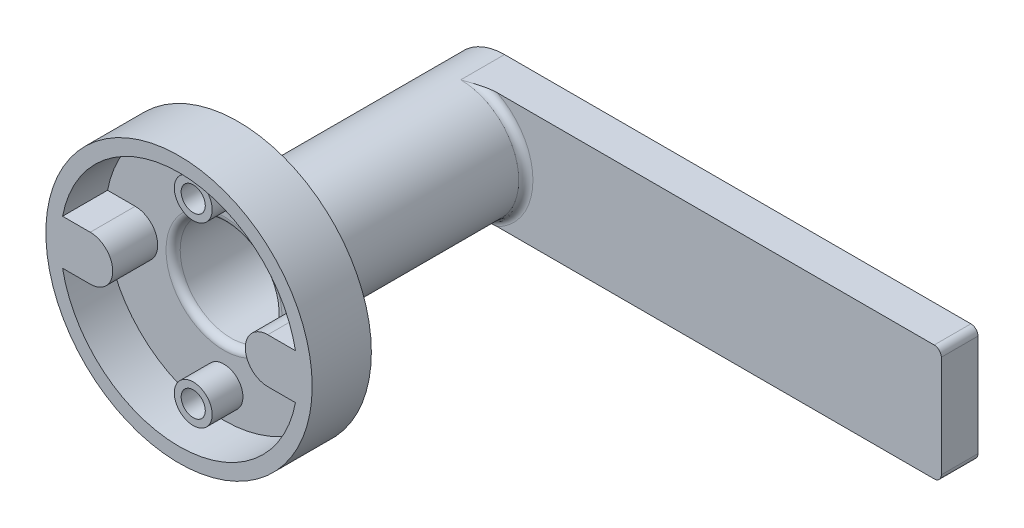
ISO-10303-21;
HEADER;
FILE_DESCRIPTION(('STEP AP214'),'2;1');
FILE_NAME('part.step','',(''),(''),'','','');
FILE_SCHEMA(('AUTOMOTIVE_DESIGN { 1 0 10303 214 1 1 1 1 }'));
ENDSEC;
DATA;
#1=APPLICATION_CONTEXT('core data for automotive mechanical design processes');
#2=APPLICATION_PROTOCOL_DEFINITION('international standard','automotive_design',2000,#1);
#3=PRODUCT_CONTEXT('',#1,'mechanical');
#4=PRODUCT('Part','Part','',(#3));
#5=PRODUCT_RELATED_PRODUCT_CATEGORY('part','',(#4));
#6=PRODUCT_DEFINITION_FORMATION('','',#4);
#7=PRODUCT_DEFINITION_CONTEXT('part definition',#1,'design');
#8=PRODUCT_DEFINITION('design','',#6,#7);
#9=PRODUCT_DEFINITION_SHAPE('','',#8);
#10=(LENGTH_UNIT() NAMED_UNIT(*) SI_UNIT(.MILLI.,.METRE.));
#11=(NAMED_UNIT(*) PLANE_ANGLE_UNIT() SI_UNIT($,.RADIAN.));
#12=(NAMED_UNIT(*) SI_UNIT($,.STERADIAN.) SOLID_ANGLE_UNIT());
#13=UNCERTAINTY_MEASURE_WITH_UNIT(LENGTH_MEASURE(1.E-05),#10,'distance_accuracy_value','');
#14=(GEOMETRIC_REPRESENTATION_CONTEXT(3) GLOBAL_UNCERTAINTY_ASSIGNED_CONTEXT((#13)) GLOBAL_UNIT_ASSIGNED_CONTEXT((#10,
#11,#12)) REPRESENTATION_CONTEXT('',''));
#15=CARTESIAN_POINT('',(0.,0.,0.));
#16=DIRECTION('',(0.,0.,1.));
#17=DIRECTION('',(1.,0.,0.));
#18=AXIS2_PLACEMENT_3D('',#15,#16,#17);
#19=CARTESIAN_POINT('',(0.,0.,12.7));
#20=DIRECTION('',(0.,0.,-1.));
#21=DIRECTION('',(-1.,0.,0.));
#22=AXIS2_PLACEMENT_3D('',#19,#20,#21);
#23=CYLINDRICAL_SURFACE('',#22,28.575);
#24=CARTESIAN_POINT('',(0.,0.,12.7));
#25=DIRECTION('',(0.,0.,1.));
#26=DIRECTION('',(1.,0.,0.));
#27=AXIS2_PLACEMENT_3D('',#24,#25,#26);
#28=CIRCLE('',#27,28.575);
#29=CARTESIAN_POINT('',(28.575,0.,12.7));
#30=VERTEX_POINT('',#29);
#31=EDGE_CURVE('E279',#30,#30,#28,.T.);
#32=ORIENTED_EDGE('',*,*,#31,.F.);
#33=EDGE_LOOP('',(#32));
#34=FACE_BOUND('',#33,.T.);
#35=CARTESIAN_POINT('',(0.,0.,0.));
#36=DIRECTION('',(0.,0.,1.));
#37=DIRECTION('',(1.,0.,0.));
#38=AXIS2_PLACEMENT_3D('',#35,#36,#37);
#39=CIRCLE('',#38,28.575);
#40=CARTESIAN_POINT('',(28.575,0.,0.));
#41=VERTEX_POINT('',#40);
#42=EDGE_CURVE('E263',#41,#41,#39,.T.);
#43=ORIENTED_EDGE('',*,*,#42,.T.);
#44=EDGE_LOOP('',(#43));
#45=FACE_BOUND('',#44,.T.);
#46=ADVANCED_FACE('F41',(#34,#45),#23,.T.);
#47=CARTESIAN_POINT('',(0.,0.,12.7));
#48=DIRECTION('',(0.,0.,1.));
#49=DIRECTION('',(1.,0.,0.));
#50=AXIS2_PLACEMENT_3D('',#47,#48,#49);
#51=PLANE('',#50);
#52=CARTESIAN_POINT('',(19.05,0.,12.7));
#53=DIRECTION('',(0.,0.,-1.));
#54=DIRECTION('',(-1.,0.,0.));
#55=AXIS2_PLACEMENT_3D('',#52,#53,#54);
#56=CIRCLE('',#55,4.826);
#57=CARTESIAN_POINT('',(19.05,-4.826,12.7));
#58=VERTEX_POINT('',#57);
#59=CARTESIAN_POINT('',(19.05,4.826,12.7));
#60=VERTEX_POINT('',#59);
#61=EDGE_CURVE('E214',#58,#60,#56,.T.);
#62=ORIENTED_EDGE('',*,*,#61,.F.);
#63=DIRECTION('',(-1.,0.,0.));
#64=VECTOR('',#63,1.);
#65=CARTESIAN_POINT('',(19.05,-4.826,12.7));
#66=LINE('',#65,#64);
#67=CARTESIAN_POINT('',(24.9900993985777,-4.826,12.7));
#68=VERTEX_POINT('',#67);
#69=EDGE_CURVE('E218',#68,#58,#66,.T.);
#70=ORIENTED_EDGE('',*,*,#69,.F.);
#71=CARTESIAN_POINT('',(0.,0.,12.7));
#72=DIRECTION('',(0.,0.,1.));
#73=DIRECTION('',(1.,0.,0.));
#74=AXIS2_PLACEMENT_3D('',#71,#72,#73);
#75=CIRCLE('',#74,25.451823980823);
#76=CARTESIAN_POINT('',(-24.9900993985777,-4.82599999999999,12.7));
#77=VERTEX_POINT('',#76);
#78=EDGE_CURVE('E257',#77,#68,#75,.T.);
#79=ORIENTED_EDGE('',*,*,#78,.F.);
#80=DIRECTION('',(-1.,0.,0.));
#81=VECTOR('',#80,1.);
#82=CARTESIAN_POINT('',(-19.05,-4.826,12.7));
#83=LINE('',#82,#81);
#84=CARTESIAN_POINT('',(-19.05,-4.826,12.7));
#85=VERTEX_POINT('',#84);
#86=EDGE_CURVE('E254',#85,#77,#83,.T.);
#87=ORIENTED_EDGE('',*,*,#86,.F.);
#88=CARTESIAN_POINT('',(-19.05,0.,12.7));
#89=DIRECTION('',(0.,0.,-1.));
#90=DIRECTION('',(1.,0.,0.));
#91=AXIS2_PLACEMENT_3D('',#88,#89,#90);
#92=CIRCLE('',#91,4.826);
#93=CARTESIAN_POINT('',(-19.05,4.826,12.7));
#94=VERTEX_POINT('',#93);
#95=EDGE_CURVE('E249',#94,#85,#92,.T.);
#96=ORIENTED_EDGE('',*,*,#95,.F.);
#97=DIRECTION('',(1.,0.,0.));
#98=VECTOR('',#97,1.);
#99=CARTESIAN_POINT('',(-19.05,4.826,12.7));
#100=LINE('',#99,#98);
#101=CARTESIAN_POINT('',(-24.9900993985777,4.826,12.7));
#102=VERTEX_POINT('',#101);
#103=EDGE_CURVE('E250',#102,#94,#100,.T.);
#104=ORIENTED_EDGE('',*,*,#103,.F.);
#105=CARTESIAN_POINT('',(0.,0.,12.7));
#106=DIRECTION('',(0.,0.,1.));
#107=DIRECTION('',(1.,0.,0.));
#108=AXIS2_PLACEMENT_3D('',#105,#106,#107);
#109=CIRCLE('',#108,25.451823980823);
#110=CARTESIAN_POINT('',(24.9900993985777,4.826,12.7));
#111=VERTEX_POINT('',#110);
#112=EDGE_CURVE('E242',#111,#102,#109,.T.);
#113=ORIENTED_EDGE('',*,*,#112,.F.);
#114=DIRECTION('',(1.,0.,0.));
#115=VECTOR('',#114,1.);
#116=CARTESIAN_POINT('',(19.05,4.826,12.7));
#117=LINE('',#116,#115);
#118=EDGE_CURVE('E241',#60,#111,#117,.T.);
#119=ORIENTED_EDGE('',*,*,#118,.F.);
#120=EDGE_LOOP('',(#62,#70,#79,#87,#96,#104,#113,#119));
#121=FACE_BOUND('',#120,.T.);
#122=ORIENTED_EDGE('',*,*,#31,.T.);
#123=EDGE_LOOP('',(#122));
#124=FACE_BOUND('',#123,.T.);
#125=ADVANCED_FACE('F344',(#121,#124),#51,.T.);
#126=CARTESIAN_POINT('',(0.,0.,0.));
#127=DIRECTION('',(0.,0.,1.));
#128=DIRECTION('',(1.,0.,0.));
#129=AXIS2_PLACEMENT_3D('',#126,#127,#128);
#130=PLANE('',#129);
#131=CARTESIAN_POINT('',(0.,0.,0.));
#132=DIRECTION('',(0.,0.,1.));
#133=DIRECTION('',(1.,0.,0.));
#134=AXIS2_PLACEMENT_3D('',#131,#132,#133);
#135=CIRCLE('',#134,12.446);
#136=CARTESIAN_POINT('',(12.446,0.,0.));
#137=VERTEX_POINT('',#136);
#138=EDGE_CURVE('E288',#137,#137,#135,.F.);
#139=ORIENTED_EDGE('',*,*,#138,.F.);
#140=EDGE_LOOP('',(#139));
#141=FACE_BOUND('',#140,.T.);
#142=CARTESIAN_POINT('',(0.,19.05,0.));
#143=DIRECTION('',(0.,0.,1.));
#144=DIRECTION('',(1.,0.,0.));
#145=AXIS2_PLACEMENT_3D('',#142,#143,#144);
#146=CIRCLE('',#145,2.59079999999999);
#147=CARTESIAN_POINT('',(2.59079999999999,19.05,0.));
#148=VERTEX_POINT('',#147);
#149=EDGE_CURVE('E198',#148,#148,#146,.T.);
#150=ORIENTED_EDGE('',*,*,#149,.T.);
#151=EDGE_LOOP('',(#150));
#152=FACE_BOUND('',#151,.T.);
#153=CARTESIAN_POINT('',(0.,-19.05,0.));
#154=DIRECTION('',(0.,0.,1.));
#155=DIRECTION('',(1.,0.,0.));
#156=AXIS2_PLACEMENT_3D('',#153,#154,#155);
#157=CIRCLE('',#156,2.59079999999999);
#158=CARTESIAN_POINT('',(2.59079999999999,-19.05,0.));
#159=VERTEX_POINT('',#158);
#160=EDGE_CURVE('E203',#159,#159,#157,.T.);
#161=ORIENTED_EDGE('',*,*,#160,.T.);
#162=EDGE_LOOP('',(#161));
#163=FACE_BOUND('',#162,.T.);
#164=ORIENTED_EDGE('',*,*,#42,.F.);
#165=EDGE_LOOP('',(#164));
#166=FACE_BOUND('',#165,.T.);
#167=ADVANCED_FACE('F348',(#141,#152,#163,#166),#130,.F.);
#168=CARTESIAN_POINT('',(19.05,0.,3.048));
#169=DIRECTION('',(0.,0.,1.));
#170=DIRECTION('',(1.,0.,0.));
#171=AXIS2_PLACEMENT_3D('',#168,#169,#170);
#172=CYLINDRICAL_SURFACE('',#171,4.826);
#173=ORIENTED_EDGE('',*,*,#61,.T.);
#174=DIRECTION('',(0.,0.,1.));
#175=VECTOR('',#174,1.);
#176=CARTESIAN_POINT('',(19.05,4.826,3.048));
#177=LINE('',#176,#175);
#178=CARTESIAN_POINT('',(19.05,4.826,3.048));
#179=VERTEX_POINT('',#178);
#180=EDGE_CURVE('E237',#179,#60,#177,.T.);
#181=ORIENTED_EDGE('',*,*,#180,.F.);
#182=CARTESIAN_POINT('',(19.05,0.,3.048));
#183=DIRECTION('',(0.,0.,-1.));
#184=DIRECTION('',(-1.,0.,0.));
#185=AXIS2_PLACEMENT_3D('',#182,#183,#184);
#186=CIRCLE('',#185,4.826);
#187=CARTESIAN_POINT('',(19.05,-4.826,3.048));
#188=VERTEX_POINT('',#187);
#189=EDGE_CURVE('E211',#188,#179,#186,.T.);
#190=ORIENTED_EDGE('',*,*,#189,.F.);
#191=DIRECTION('',(0.,0.,1.));
#192=VECTOR('',#191,1.);
#193=CARTESIAN_POINT('',(19.05,-4.826,3.048));
#194=LINE('',#193,#192);
#195=EDGE_CURVE('E262',#188,#58,#194,.T.);
#196=ORIENTED_EDGE('',*,*,#195,.T.);
#197=EDGE_LOOP('',(#173,#181,#190,#196));
#198=FACE_BOUND('',#197,.T.);
#199=ADVANCED_FACE('F358',(#198),#172,.T.);
#200=CARTESIAN_POINT('',(19.05,-4.826,3.048));
#201=DIRECTION('',(0.,1.,0.));
#202=DIRECTION('',(-1.,0.,0.));
#203=AXIS2_PLACEMENT_3D('',#200,#201,#202);
#204=PLANE('',#203);
#205=ORIENTED_EDGE('',*,*,#69,.T.);
#206=ORIENTED_EDGE('',*,*,#195,.F.);
#207=DIRECTION('',(-1.,0.,0.));
#208=VECTOR('',#207,1.);
#209=CARTESIAN_POINT('',(19.05,-4.826,3.048));
#210=LINE('',#209,#208);
#211=CARTESIAN_POINT('',(24.9900993985777,-4.826,3.048));
#212=VERTEX_POINT('',#211);
#213=EDGE_CURVE('E236',#212,#188,#210,.T.);
#214=ORIENTED_EDGE('',*,*,#213,.F.);
#215=DIRECTION('',(0.,0.,1.));
#216=VECTOR('',#215,1.);
#217=CARTESIAN_POINT('',(24.9900993985777,-4.826,3.048));
#218=LINE('',#217,#216);
#219=EDGE_CURVE('E264',#212,#68,#218,.T.);
#220=ORIENTED_EDGE('',*,*,#219,.T.);
#221=EDGE_LOOP('',(#205,#206,#214,#220));
#222=FACE_BOUND('',#221,.T.);
#223=ADVANCED_FACE('F361',(#222),#204,.F.);
#224=CARTESIAN_POINT('',(0.,0.,3.048));
#225=DIRECTION('',(0.,0.,1.));
#226=DIRECTION('',(1.,0.,0.));
#227=AXIS2_PLACEMENT_3D('',#224,#225,#226);
#228=CYLINDRICAL_SURFACE('',#227,25.451823980823);
#229=ORIENTED_EDGE('',*,*,#78,.T.);
#230=ORIENTED_EDGE('',*,*,#219,.F.);
#231=CARTESIAN_POINT('',(0.,0.,3.048));
#232=DIRECTION('',(0.,0.,1.));
#233=DIRECTION('',(1.,0.,0.));
#234=AXIS2_PLACEMENT_3D('',#231,#232,#233);
#235=CIRCLE('',#234,25.451823980823);
#236=CARTESIAN_POINT('',(-24.9900993985777,-4.82599999999999,3.048));
#237=VERTEX_POINT('',#236);
#238=EDGE_CURVE('E231',#237,#212,#235,.T.);
#239=ORIENTED_EDGE('',*,*,#238,.F.);
#240=DIRECTION('',(0.,0.,1.));
#241=VECTOR('',#240,1.);
#242=CARTESIAN_POINT('',(-24.9900993985777,-4.82599999999999,3.048));
#243=LINE('',#242,#241);
#244=EDGE_CURVE('E269',#237,#77,#243,.T.);
#245=ORIENTED_EDGE('',*,*,#244,.T.);
#246=EDGE_LOOP('',(#229,#230,#239,#245));
#247=FACE_BOUND('',#246,.T.);
#248=ADVANCED_FACE('F386',(#247),#228,.F.);
#249=CARTESIAN_POINT('',(-19.05,-4.826,3.048));
#250=DIRECTION('',(0.,1.,0.));
#251=DIRECTION('',(-1.,0.,0.));
#252=AXIS2_PLACEMENT_3D('',#249,#250,#251);
#253=PLANE('',#252);
#254=ORIENTED_EDGE('',*,*,#86,.T.);
#255=ORIENTED_EDGE('',*,*,#244,.F.);
#256=DIRECTION('',(-1.,0.,0.));
#257=VECTOR('',#256,1.);
#258=CARTESIAN_POINT('',(-19.05,-4.826,3.048));
#259=LINE('',#258,#257);
#260=CARTESIAN_POINT('',(-19.05,-4.826,3.048));
#261=VERTEX_POINT('',#260);
#262=EDGE_CURVE('E229',#261,#237,#259,.T.);
#263=ORIENTED_EDGE('',*,*,#262,.F.);
#264=DIRECTION('',(0.,0.,1.));
#265=VECTOR('',#264,1.);
#266=CARTESIAN_POINT('',(-19.05,-4.826,3.048));
#267=LINE('',#266,#265);
#268=EDGE_CURVE('E270',#261,#85,#267,.T.);
#269=ORIENTED_EDGE('',*,*,#268,.T.);
#270=EDGE_LOOP('',(#254,#255,#263,#269));
#271=FACE_BOUND('',#270,.T.);
#272=ADVANCED_FACE('F383',(#271),#253,.F.);
#273=CARTESIAN_POINT('',(-19.05,0.,3.048));
#274=DIRECTION('',(0.,0.,1.));
#275=DIRECTION('',(1.,0.,0.));
#276=AXIS2_PLACEMENT_3D('',#273,#274,#275);
#277=CYLINDRICAL_SURFACE('',#276,4.826);
#278=ORIENTED_EDGE('',*,*,#95,.T.);
#279=ORIENTED_EDGE('',*,*,#268,.F.);
#280=CARTESIAN_POINT('',(-19.05,0.,3.048));
#281=DIRECTION('',(0.,0.,-1.));
#282=DIRECTION('',(1.,0.,0.));
#283=AXIS2_PLACEMENT_3D('',#280,#281,#282);
#284=CIRCLE('',#283,4.826);
#285=CARTESIAN_POINT('',(-19.05,4.826,3.048));
#286=VERTEX_POINT('',#285);
#287=EDGE_CURVE('E227',#286,#261,#284,.T.);
#288=ORIENTED_EDGE('',*,*,#287,.F.);
#289=DIRECTION('',(0.,0.,1.));
#290=VECTOR('',#289,1.);
#291=CARTESIAN_POINT('',(-19.05,4.826,3.048));
#292=LINE('',#291,#290);
#293=EDGE_CURVE('E267',#286,#94,#292,.T.);
#294=ORIENTED_EDGE('',*,*,#293,.T.);
#295=EDGE_LOOP('',(#278,#279,#288,#294));
#296=FACE_BOUND('',#295,.T.);
#297=ADVANCED_FACE('F382',(#296),#277,.T.);
#298=CARTESIAN_POINT('',(-19.05,4.826,3.048));
#299=DIRECTION('',(0.,-1.,0.));
#300=DIRECTION('',(1.,0.,0.));
#301=AXIS2_PLACEMENT_3D('',#298,#299,#300);
#302=PLANE('',#301);
#303=ORIENTED_EDGE('',*,*,#103,.T.);
#304=ORIENTED_EDGE('',*,*,#293,.F.);
#305=DIRECTION('',(1.,0.,0.));
#306=VECTOR('',#305,1.);
#307=CARTESIAN_POINT('',(-19.05,4.826,3.048));
#308=LINE('',#307,#306);
#309=CARTESIAN_POINT('',(-24.9900993985777,4.826,3.048));
#310=VERTEX_POINT('',#309);
#311=EDGE_CURVE('E223',#310,#286,#308,.T.);
#312=ORIENTED_EDGE('',*,*,#311,.F.);
#313=DIRECTION('',(0.,0.,1.));
#314=VECTOR('',#313,1.);
#315=CARTESIAN_POINT('',(-24.9900993985777,4.826,3.048));
#316=LINE('',#315,#314);
#317=EDGE_CURVE('E275',#310,#102,#316,.T.);
#318=ORIENTED_EDGE('',*,*,#317,.T.);
#319=EDGE_LOOP('',(#303,#304,#312,#318));
#320=FACE_BOUND('',#319,.T.);
#321=ADVANCED_FACE('F380',(#320),#302,.F.);
#322=CARTESIAN_POINT('',(0.,0.,3.048));
#323=DIRECTION('',(0.,0.,1.));
#324=DIRECTION('',(1.,0.,0.));
#325=AXIS2_PLACEMENT_3D('',#322,#323,#324);
#326=CYLINDRICAL_SURFACE('',#325,25.451823980823);
#327=ORIENTED_EDGE('',*,*,#112,.T.);
#328=ORIENTED_EDGE('',*,*,#317,.F.);
#329=CARTESIAN_POINT('',(0.,0.,3.048));
#330=DIRECTION('',(0.,0.,1.));
#331=DIRECTION('',(1.,0.,0.));
#332=AXIS2_PLACEMENT_3D('',#329,#330,#331);
#333=CIRCLE('',#332,25.451823980823);
#334=CARTESIAN_POINT('',(24.9900993985777,4.826,3.048));
#335=VERTEX_POINT('',#334);
#336=EDGE_CURVE('E224',#335,#310,#333,.T.);
#337=ORIENTED_EDGE('',*,*,#336,.F.);
#338=DIRECTION('',(0.,0.,1.));
#339=VECTOR('',#338,1.);
#340=CARTESIAN_POINT('',(24.9900993985777,4.826,3.048));
#341=LINE('',#340,#339);
#342=EDGE_CURVE('E274',#335,#111,#341,.T.);
#343=ORIENTED_EDGE('',*,*,#342,.T.);
#344=EDGE_LOOP('',(#327,#328,#337,#343));
#345=FACE_BOUND('',#344,.T.);
#346=ADVANCED_FACE('F373',(#345),#326,.F.);
#347=CARTESIAN_POINT('',(19.05,4.826,3.048));
#348=DIRECTION('',(0.,-1.,0.));
#349=DIRECTION('',(1.,0.,0.));
#350=AXIS2_PLACEMENT_3D('',#347,#348,#349);
#351=PLANE('',#350);
#352=ORIENTED_EDGE('',*,*,#118,.T.);
#353=ORIENTED_EDGE('',*,*,#342,.F.);
#354=DIRECTION('',(1.,0.,0.));
#355=VECTOR('',#354,1.);
#356=CARTESIAN_POINT('',(19.05,4.826,3.048));
#357=LINE('',#356,#355);
#358=EDGE_CURVE('E220',#179,#335,#357,.T.);
#359=ORIENTED_EDGE('',*,*,#358,.F.);
#360=ORIENTED_EDGE('',*,*,#180,.T.);
#361=EDGE_LOOP('',(#352,#353,#359,#360));
#362=FACE_BOUND('',#361,.T.);
#363=ADVANCED_FACE('F367',(#362),#351,.F.);
#364=CARTESIAN_POINT('',(19.05,0.,3.048));
#365=DIRECTION('',(0.,0.,-1.));
#366=DIRECTION('',(-1.,0.,0.));
#367=AXIS2_PLACEMENT_3D('',#364,#365,#366);
#368=PLANE('',#367);
#369=CARTESIAN_POINT('',(0.,0.,3.048));
#370=DIRECTION('',(0.,0.,-1.));
#371=DIRECTION('',(-1.,0.,0.));
#372=AXIS2_PLACEMENT_3D('',#369,#370,#371);
#373=CIRCLE('',#372,12.446);
#374=CARTESIAN_POINT('',(-12.446,0.,3.048));
#375=VERTEX_POINT('',#374);
#376=EDGE_CURVE('E302',#375,#375,#373,.T.);
#377=ORIENTED_EDGE('',*,*,#376,.T.);
#378=EDGE_LOOP('',(#377));
#379=FACE_BOUND('',#378,.T.);
#380=CARTESIAN_POINT('',(0.,-19.05,3.048));
#381=DIRECTION('',(0.,0.,-1.));
#382=DIRECTION('',(-1.,0.,0.));
#383=AXIS2_PLACEMENT_3D('',#380,#381,#382);
#384=CIRCLE('',#383,4.064);
#385=CARTESIAN_POINT('',(-4.064,-19.05,3.048));
#386=VERTEX_POINT('',#385);
#387=EDGE_CURVE('E289',#386,#386,#384,.F.);
#388=ORIENTED_EDGE('',*,*,#387,.F.);
#389=EDGE_LOOP('',(#388));
#390=FACE_BOUND('',#389,.T.);
#391=CARTESIAN_POINT('',(0.,19.05,3.048));
#392=DIRECTION('',(0.,0.,-1.));
#393=DIRECTION('',(-1.,0.,0.));
#394=AXIS2_PLACEMENT_3D('',#391,#392,#393);
#395=CIRCLE('',#394,4.064);
#396=CARTESIAN_POINT('',(-4.064,19.05,3.048));
#397=VERTEX_POINT('',#396);
#398=EDGE_CURVE('E282',#397,#397,#395,.F.);
#399=ORIENTED_EDGE('',*,*,#398,.F.);
#400=EDGE_LOOP('',(#399));
#401=FACE_BOUND('',#400,.T.);
#402=ORIENTED_EDGE('',*,*,#189,.T.);
#403=ORIENTED_EDGE('',*,*,#358,.T.);
#404=ORIENTED_EDGE('',*,*,#336,.T.);
#405=ORIENTED_EDGE('',*,*,#311,.T.);
#406=ORIENTED_EDGE('',*,*,#287,.T.);
#407=ORIENTED_EDGE('',*,*,#262,.T.);
#408=ORIENTED_EDGE('',*,*,#238,.T.);
#409=ORIENTED_EDGE('',*,*,#213,.T.);
#410=EDGE_LOOP('',(#402,#403,#404,#405,#406,#407,#408,#409));
#411=FACE_BOUND('',#410,.T.);
#412=ADVANCED_FACE('F375',(#379,#390,#401,#411),#368,.F.);
#413=CARTESIAN_POINT('',(0.,19.05,24.1947278349685));
#414=DIRECTION('',(0.,0.,-1.));
#415=DIRECTION('',(-1.,0.,0.));
#416=AXIS2_PLACEMENT_3D('',#413,#414,#415);
#417=CYLINDRICAL_SURFACE('',#416,4.064);
#418=ORIENTED_EDGE('',*,*,#398,.T.);
#419=EDGE_LOOP('',(#418));
#420=FACE_BOUND('',#419,.T.);
#421=CARTESIAN_POINT('',(0.,19.05,9.652));
#422=DIRECTION('',(0.,0.,1.));
#423=DIRECTION('',(1.,0.,0.));
#424=AXIS2_PLACEMENT_3D('',#421,#422,#423);
#425=CIRCLE('',#424,4.064);
#426=CARTESIAN_POINT('',(4.064,19.05,9.652));
#427=VERTEX_POINT('',#426);
#428=EDGE_CURVE('E208',#427,#427,#425,.T.);
#429=ORIENTED_EDGE('',*,*,#428,.F.);
#430=EDGE_LOOP('',(#429));
#431=FACE_BOUND('',#430,.T.);
#432=ADVANCED_FACE('F398',(#420,#431),#417,.T.);
#433=CARTESIAN_POINT('',(0.,0.,9.652));
#434=DIRECTION('',(0.,0.,1.));
#435=DIRECTION('',(1.,0.,0.));
#436=AXIS2_PLACEMENT_3D('',#433,#434,#435);
#437=PLANE('',#436);
#438=CARTESIAN_POINT('',(0.,19.05,9.652));
#439=DIRECTION('',(0.,0.,1.));
#440=DIRECTION('',(1.,0.,0.));
#441=AXIS2_PLACEMENT_3D('',#438,#439,#440);
#442=CIRCLE('',#441,2.59079999999999);
#443=CARTESIAN_POINT('',(2.59079999999999,19.05,9.652));
#444=VERTEX_POINT('',#443);
#445=EDGE_CURVE('E193',#444,#444,#442,.T.);
#446=ORIENTED_EDGE('',*,*,#445,.F.);
#447=EDGE_LOOP('',(#446));
#448=FACE_BOUND('',#447,.T.);
#449=ORIENTED_EDGE('',*,*,#428,.T.);
#450=EDGE_LOOP('',(#449));
#451=FACE_BOUND('',#450,.T.);
#452=ADVANCED_FACE('F402',(#448,#451),#437,.T.);
#453=CARTESIAN_POINT('',(0.,-19.05,24.1947278349685));
#454=DIRECTION('',(0.,0.,-1.));
#455=DIRECTION('',(-1.,0.,0.));
#456=AXIS2_PLACEMENT_3D('',#453,#454,#455);
#457=CYLINDRICAL_SURFACE('',#456,4.064);
#458=ORIENTED_EDGE('',*,*,#387,.T.);
#459=EDGE_LOOP('',(#458));
#460=FACE_BOUND('',#459,.T.);
#461=CARTESIAN_POINT('',(0.,-19.05,9.652));
#462=DIRECTION('',(0.,0.,1.));
#463=DIRECTION('',(1.,0.,0.));
#464=AXIS2_PLACEMENT_3D('',#461,#462,#463);
#465=CIRCLE('',#464,4.064);
#466=CARTESIAN_POINT('',(4.064,-19.05,9.652));
#467=VERTEX_POINT('',#466);
#468=EDGE_CURVE('E210',#467,#467,#465,.T.);
#469=ORIENTED_EDGE('',*,*,#468,.F.);
#470=EDGE_LOOP('',(#469));
#471=FACE_BOUND('',#470,.T.);
#472=ADVANCED_FACE('F404',(#460,#471),#457,.T.);
#473=CARTESIAN_POINT('',(0.,0.,9.652));
#474=DIRECTION('',(0.,0.,1.));
#475=DIRECTION('',(1.,0.,0.));
#476=AXIS2_PLACEMENT_3D('',#473,#474,#475);
#477=PLANE('',#476);
#478=CARTESIAN_POINT('',(0.,-19.05,9.652));
#479=DIRECTION('',(0.,0.,1.));
#480=DIRECTION('',(1.,0.,0.));
#481=AXIS2_PLACEMENT_3D('',#478,#479,#480);
#482=CIRCLE('',#481,2.59079999999999);
#483=CARTESIAN_POINT('',(2.59079999999999,-19.05,9.652));
#484=VERTEX_POINT('',#483);
#485=EDGE_CURVE('E204',#484,#484,#482,.T.);
#486=ORIENTED_EDGE('',*,*,#485,.F.);
#487=EDGE_LOOP('',(#486));
#488=FACE_BOUND('',#487,.T.);
#489=ORIENTED_EDGE('',*,*,#468,.T.);
#490=EDGE_LOOP('',(#489));
#491=FACE_BOUND('',#490,.T.);
#492=ADVANCED_FACE('F406',(#488,#491),#477,.T.);
#493=CARTESIAN_POINT('',(0.,-19.05,9.652));
#494=DIRECTION('',(0.,0.,1.));
#495=DIRECTION('',(1.,0.,0.));
#496=AXIS2_PLACEMENT_3D('',#493,#494,#495);
#497=CYLINDRICAL_SURFACE('',#496,2.59079999999999);
#498=ORIENTED_EDGE('',*,*,#485,.T.);
#499=EDGE_LOOP('',(#498));
#500=FACE_BOUND('',#499,.T.);
#501=ORIENTED_EDGE('',*,*,#160,.F.);
#502=EDGE_LOOP('',(#501));
#503=FACE_BOUND('',#502,.T.);
#504=ADVANCED_FACE('F415',(#500,#503),#497,.F.);
#505=CARTESIAN_POINT('',(0.,19.05,9.652));
#506=DIRECTION('',(0.,0.,1.));
#507=DIRECTION('',(1.,0.,0.));
#508=AXIS2_PLACEMENT_3D('',#505,#506,#507);
#509=CYLINDRICAL_SURFACE('',#508,2.59079999999999);
#510=ORIENTED_EDGE('',*,*,#445,.T.);
#511=EDGE_LOOP('',(#510));
#512=FACE_BOUND('',#511,.T.);
#513=ORIENTED_EDGE('',*,*,#149,.F.);
#514=EDGE_LOOP('',(#513));
#515=FACE_BOUND('',#514,.T.);
#516=ADVANCED_FACE('F418',(#512,#515),#509,.F.);
#517=CARTESIAN_POINT('',(0.,0.,-49.276));
#518=DIRECTION('',(0.,0.,1.));
#519=DIRECTION('',(1.,0.,0.));
#520=AXIS2_PLACEMENT_3D('',#517,#518,#519);
#521=CYLINDRICAL_SURFACE('',#520,12.446);
#522=DIRECTION('',(0.,0.,1.));
#523=VECTOR('',#522,1.);
#524=CARTESIAN_POINT('',(0.,-12.446,-57.15));
#525=LINE('',#524,#523);
#526=CARTESIAN_POINT('',(0.,-12.446,-57.15));
#527=VERTEX_POINT('',#526);
#528=CARTESIAN_POINT('',(0.,-12.446,-47.752));
#529=VERTEX_POINT('',#528);
#530=EDGE_CURVE('E167',#527,#529,#525,.T.);
#531=ORIENTED_EDGE('',*,*,#530,.T.);
#532=CARTESIAN_POINT('',(0.,0.,-47.752));
#533=DIRECTION('',(0.,0.,-1.));
#534=DIRECTION('',(-1.,0.,0.));
#535=AXIS2_PLACEMENT_3D('',#532,#533,#534);
#536=CIRCLE('',#535,12.446);
#537=CARTESIAN_POINT('',(0.,12.446,-47.752));
#538=VERTEX_POINT('',#537);
#539=EDGE_CURVE('E299',#529,#538,#536,.F.);
#540=ORIENTED_EDGE('',*,*,#539,.T.);
#541=DIRECTION('',(0.,0.,1.));
#542=VECTOR('',#541,1.);
#543=CARTESIAN_POINT('',(0.,12.446,-57.15));
#544=LINE('',#543,#542);
#545=CARTESIAN_POINT('',(0.,12.446,-57.15));
#546=VERTEX_POINT('',#545);
#547=EDGE_CURVE('E180',#546,#538,#544,.T.);
#548=ORIENTED_EDGE('',*,*,#547,.F.);
#549=CARTESIAN_POINT('',(0.,0.,-57.15));
#550=DIRECTION('',(0.,0.,-1.));
#551=DIRECTION('',(-1.,0.,0.));
#552=AXIS2_PLACEMENT_3D('',#549,#550,#551);
#553=CIRCLE('',#552,12.446);
#554=EDGE_CURVE('E157',#527,#546,#553,.T.);
#555=ORIENTED_EDGE('',*,*,#554,.F.);
#556=EDGE_LOOP('',(#531,#540,#548,#555));
#557=FACE_BOUND('',#556,.T.);
#558=ORIENTED_EDGE('',*,*,#138,.T.);
#559=EDGE_LOOP('',(#558));
#560=FACE_BOUND('',#559,.T.);
#561=ADVANCED_FACE('F177',(#557,#560),#521,.T.);
#562=CARTESIAN_POINT('',(0.,0.,-80.1680810564779));
#563=DIRECTION('',(0.,0.,1.));
#564=DIRECTION('',(1.,0.,0.));
#565=AXIS2_PLACEMENT_3D('',#562,#563,#564);
#566=CYLINDRICAL_SURFACE('',#565,10.922);
#567=CARTESIAN_POINT('',(0.,0.,1.524));
#568=DIRECTION('',(0.,0.,-1.));
#569=DIRECTION('',(-1.,0.,0.));
#570=AXIS2_PLACEMENT_3D('',#567,#568,#569);
#571=CIRCLE('',#570,10.922);
#572=CARTESIAN_POINT('',(-10.922,0.,1.524));
#573=VERTEX_POINT('',#572);
#574=EDGE_CURVE('E301',#573,#573,#571,.F.);
#575=ORIENTED_EDGE('',*,*,#574,.T.);
#576=EDGE_LOOP('',(#575));
#577=FACE_BOUND('',#576,.T.);
#578=CARTESIAN_POINT('',(0.,0.,-49.276));
#579=DIRECTION('',(0.,0.,-1.));
#580=DIRECTION('',(-1.,0.,0.));
#581=AXIS2_PLACEMENT_3D('',#578,#579,#580);
#582=CIRCLE('',#581,10.922);
#583=CARTESIAN_POINT('',(-10.922,0.,-49.276));
#584=VERTEX_POINT('',#583);
#585=EDGE_CURVE('E176',#584,#584,#582,.F.);
#586=ORIENTED_EDGE('',*,*,#585,.F.);
#587=EDGE_LOOP('',(#586));
#588=FACE_BOUND('',#587,.T.);
#589=ADVANCED_FACE('F424',(#577,#588),#566,.F.);
#590=CARTESIAN_POINT('',(0.,0.,-57.15));
#591=DIRECTION('',(0.,0.,-1.));
#592=DIRECTION('',(-1.,0.,0.));
#593=AXIS2_PLACEMENT_3D('',#590,#591,#592);
#594=PLANE('',#593);
#595=DIRECTION('',(0.,-1.,0.));
#596=VECTOR('',#595,1.);
#597=CARTESIAN_POINT('',(101.6,12.446,-57.15));
#598=LINE('',#597,#596);
#599=CARTESIAN_POINT('',(101.6,10.922,-57.15));
#600=VERTEX_POINT('',#599);
#601=CARTESIAN_POINT('',(101.6,-10.922,-57.15));
#602=VERTEX_POINT('',#601);
#603=EDGE_CURVE('E170',#600,#602,#598,.T.);
#604=ORIENTED_EDGE('',*,*,#603,.T.);
#605=CARTESIAN_POINT('',(100.076,-10.922,-57.15));
#606=DIRECTION('',(0.,0.,-1.));
#607=DIRECTION('',(-1.,0.,0.));
#608=AXIS2_PLACEMENT_3D('',#605,#606,#607);
#609=CIRCLE('',#608,1.524);
#610=CARTESIAN_POINT('',(100.076,-12.446,-57.15));
#611=VERTEX_POINT('',#610);
#612=EDGE_CURVE('E161',#602,#611,#609,.T.);
#613=ORIENTED_EDGE('',*,*,#612,.T.);
#614=DIRECTION('',(-1.,0.,0.));
#615=VECTOR('',#614,1.);
#616=CARTESIAN_POINT('',(101.6,-12.446,-57.15));
#617=LINE('',#616,#615);
#618=EDGE_CURVE('E159',#611,#527,#617,.T.);
#619=ORIENTED_EDGE('',*,*,#618,.T.);
#620=ORIENTED_EDGE('',*,*,#554,.T.);
#621=DIRECTION('',(1.,0.,0.));
#622=VECTOR('',#621,1.);
#623=CARTESIAN_POINT('',(101.6,12.446,-57.15));
#624=LINE('',#623,#622);
#625=CARTESIAN_POINT('',(100.076,12.446,-57.15));
#626=VERTEX_POINT('',#625);
#627=EDGE_CURVE('E181',#546,#626,#624,.T.);
#628=ORIENTED_EDGE('',*,*,#627,.T.);
#629=CARTESIAN_POINT('',(100.076,10.922,-57.15));
#630=DIRECTION('',(0.,0.,-1.));
#631=DIRECTION('',(-1.,0.,0.));
#632=AXIS2_PLACEMENT_3D('',#629,#630,#631);
#633=CIRCLE('',#632,1.524);
#634=EDGE_CURVE('E312',#626,#600,#633,.T.);
#635=ORIENTED_EDGE('',*,*,#634,.T.);
#636=EDGE_LOOP('',(#604,#613,#619,#620,#628,#635));
#637=FACE_BOUND('',#636,.T.);
#638=ADVANCED_FACE('F160',(#637),#594,.T.);
#639=CARTESIAN_POINT('',(101.6,12.446,-57.15));
#640=DIRECTION('',(0.,-1.,0.));
#641=DIRECTION('',(0.,0.,-1.));
#642=AXIS2_PLACEMENT_3D('',#639,#640,#641);
#643=PLANE('',#642);
#644=DIRECTION('',(1.,0.,0.));
#645=VECTOR('',#644,1.);
#646=CARTESIAN_POINT('',(101.6,12.446,-49.276));
#647=LINE('',#646,#645);
#648=CARTESIAN_POINT('',(6.34491796637277,12.446,-49.276));
#649=VERTEX_POINT('',#648);
#650=CARTESIAN_POINT('',(100.076,12.446,-49.276));
#651=VERTEX_POINT('',#650);
#652=EDGE_CURVE('E188',#649,#651,#647,.T.);
#653=ORIENTED_EDGE('',*,*,#652,.T.);
#654=DIRECTION('',(0.,0.,1.));
#655=VECTOR('',#654,1.);
#656=CARTESIAN_POINT('',(100.076,12.446,-57.15));
#657=LINE('',#656,#655);
#658=EDGE_CURVE('E65',#651,#626,#657,.F.);
#659=ORIENTED_EDGE('',*,*,#658,.T.);
#660=ORIENTED_EDGE('',*,*,#627,.F.);
#661=ORIENTED_EDGE('',*,*,#547,.T.);
#662=CARTESIAN_POINT('',(6.34491796637277,12.446,-49.276));
#663=CARTESIAN_POINT('',(6.21533524094485,12.446,-49.2759732705405));
#664=CARTESIAN_POINT('',(6.08579369063811,12.446,-49.27259226928));
#665=CARTESIAN_POINT('',(5.82706524459241,12.446,-49.259910087951));
#666=CARTESIAN_POINT('',(5.6978781945778,12.446,-49.2506121205866));
#667=CARTESIAN_POINT('',(5.4402955593906,12.446,-49.2269107528351));
#668=CARTESIAN_POINT('',(5.31189882415412,12.446,-49.2125195023357));
#669=CARTESIAN_POINT('',(5.05567590714475,12.446,-49.1792496205522));
#670=CARTESIAN_POINT('',(4.92784981517291,12.446,-49.1603703067066));
#671=CARTESIAN_POINT('',(4.54726190236325,12.446,-49.0981575716032));
#672=CARTESIAN_POINT('',(4.29543863295937,12.446,-49.0490520465874));
#673=CARTESIAN_POINT('',(3.79431096207436,12.446,-48.9389015359754));
#674=CARTESIAN_POINT('',(3.54500841851374,12.446,-48.8778483354951));
#675=CARTESIAN_POINT('',(3.01979635859548,12.446,-48.7389881468602));
#676=CARTESIAN_POINT('',(2.74418711385954,12.446,-48.6600566773526));
#677=CARTESIAN_POINT('',(2.19547772469525,12.446,-48.4941969315973));
#678=CARTESIAN_POINT('',(1.92237711929461,12.446,-48.4072701582111));
#679=CARTESIAN_POINT('',(1.1047936535399,12.446,-48.1385183371954));
#680=CARTESIAN_POINT('',(0.562885676700975,12.446,-47.9489679517187));
#681=CARTESIAN_POINT('',(0.0140400977837042,12.446,-47.7569129993086));
#682=CARTESIAN_POINT('',(0.00702004561032453,12.446,-47.7544564925513));
#683=CARTESIAN_POINT('',(0.,12.446,-47.752));
#684=B_SPLINE_CURVE_WITH_KNOTS('',3,(#662,#663,#664,#665,#666,#667,#668,#669,#670,#671,#672,
#673,#674,#675,#676,#677,#678,#679,#680,#681,#682,#683),.UNSPECIFIED.,.F.,.F.,(4,2,2,2,2,2,2,2,
2,2,4),(0.,0.388645930924585,0.777081020636638,1.16459568621553,1.5521693242234,
2.32144242636155,3.09124632924267,3.95113147757733,4.81085532404043,6.5329742853189,
6.5552866137498),.UNSPECIFIED.);
#685=EDGE_CURVE('E12',#538,#649,#684,.F.);
#686=ORIENTED_EDGE('',*,*,#685,.T.);
#687=EDGE_LOOP('',(#653,#659,#660,#661,#686));
#688=FACE_BOUND('',#687,.T.);
#689=ADVANCED_FACE('F440',(#688),#643,.F.);
#690=CARTESIAN_POINT('',(101.6,-12.446,-57.15));
#691=DIRECTION('',(0.,1.,0.));
#692=DIRECTION('',(0.,0.,1.));
#693=AXIS2_PLACEMENT_3D('',#690,#691,#692);
#694=PLANE('',#693);
#695=ORIENTED_EDGE('',*,*,#618,.F.);
#696=DIRECTION('',(0.,0.,1.));
#697=VECTOR('',#696,1.);
#698=CARTESIAN_POINT('',(100.076,-12.446,-57.15));
#699=LINE('',#698,#697);
#700=CARTESIAN_POINT('',(100.076,-12.446,-49.276));
#701=VERTEX_POINT('',#700);
#702=EDGE_CURVE('E310',#611,#701,#699,.T.);
#703=ORIENTED_EDGE('',*,*,#702,.T.);
#704=DIRECTION('',(-1.,0.,0.));
#705=VECTOR('',#704,1.);
#706=CARTESIAN_POINT('',(101.6,-12.446,-49.276));
#707=LINE('',#706,#705);
#708=CARTESIAN_POINT('',(6.34491796637277,-12.446,-49.276));
#709=VERTEX_POINT('',#708);
#710=EDGE_CURVE('E189',#701,#709,#707,.T.);
#711=ORIENTED_EDGE('',*,*,#710,.T.);
#712=CARTESIAN_POINT('',(6.34491796637277,-12.446,-49.276));
#713=CARTESIAN_POINT('',(6.21533524094485,-12.446,-49.2759732705405));
#714=CARTESIAN_POINT('',(6.08579369063811,-12.446,-49.27259226928));
#715=CARTESIAN_POINT('',(5.82706524459241,-12.446,-49.259910087951));
#716=CARTESIAN_POINT('',(5.6978781945778,-12.446,-49.2506121205866));
#717=CARTESIAN_POINT('',(5.4402955593906,-12.446,-49.2269107528351));
#718=CARTESIAN_POINT('',(5.31189882415412,-12.446,-49.2125195023357));
#719=CARTESIAN_POINT('',(5.05567590714475,-12.446,-49.1792496205522));
#720=CARTESIAN_POINT('',(4.92784981517291,-12.446,-49.1603703067066));
#721=CARTESIAN_POINT('',(4.54726190236325,-12.446,-49.0981575716032));
#722=CARTESIAN_POINT('',(4.29543863295937,-12.446,-49.0490520465874));
#723=CARTESIAN_POINT('',(3.79431096207436,-12.446,-48.9389015359754));
#724=CARTESIAN_POINT('',(3.54500841851374,-12.446,-48.8778483354951));
#725=CARTESIAN_POINT('',(3.01979635859548,-12.446,-48.7389881468602));
#726=CARTESIAN_POINT('',(2.74418711385954,-12.446,-48.6600566773526));
#727=CARTESIAN_POINT('',(2.19547772469525,-12.446,-48.4941969315973));
#728=CARTESIAN_POINT('',(1.92237711929461,-12.446,-48.4072701582111));
#729=CARTESIAN_POINT('',(1.1047936535399,-12.446,-48.1385183371954));
#730=CARTESIAN_POINT('',(0.562885676700975,-12.446,-47.9489679517187));
#731=CARTESIAN_POINT('',(0.0140400977837042,-12.446,-47.7569129993086));
#732=CARTESIAN_POINT('',(0.00702004561032453,-12.446,-47.7544564925513));
#733=CARTESIAN_POINT('',(0.,-12.446,-47.752));
#734=B_SPLINE_CURVE_WITH_KNOTS('',3,(#712,#713,#714,#715,#716,#717,#718,#719,#720,#721,#722,
#723,#724,#725,#726,#727,#728,#729,#730,#731,#732,#733),.UNSPECIFIED.,.F.,.F.,(4,2,2,2,2,2,2,2,
2,2,4),(0.,0.388645930924585,0.777081020636638,1.16459568621553,1.5521693242234,
2.32144242636155,3.09124632924267,3.95113147757733,4.81085532404043,6.5329742853189,
6.5552866137498),.UNSPECIFIED.);
#735=EDGE_CURVE('E54',#709,#529,#734,.T.);
#736=ORIENTED_EDGE('',*,*,#735,.T.);
#737=ORIENTED_EDGE('',*,*,#530,.F.);
#738=EDGE_LOOP('',(#695,#703,#711,#736,#737));
#739=FACE_BOUND('',#738,.T.);
#740=ADVANCED_FACE('F171',(#739),#694,.F.);
#741=CARTESIAN_POINT('',(101.6,12.446,-57.15));
#742=DIRECTION('',(-1.,0.,0.));
#743=DIRECTION('',(0.,0.,1.));
#744=AXIS2_PLACEMENT_3D('',#741,#742,#743);
#745=PLANE('',#744);
#746=DIRECTION('',(0.,-1.,0.));
#747=VECTOR('',#746,1.);
#748=CARTESIAN_POINT('',(101.6,12.446,-49.276));
#749=LINE('',#748,#747);
#750=CARTESIAN_POINT('',(101.6,10.922,-49.276));
#751=VERTEX_POINT('',#750);
#752=CARTESIAN_POINT('',(101.6,-10.922,-49.276));
#753=VERTEX_POINT('',#752);
#754=EDGE_CURVE('E187',#751,#753,#749,.T.);
#755=ORIENTED_EDGE('',*,*,#754,.T.);
#756=DIRECTION('',(0.,0.,1.));
#757=VECTOR('',#756,1.);
#758=CARTESIAN_POINT('',(101.6,-10.922,-57.15));
#759=LINE('',#758,#757);
#760=EDGE_CURVE('E66',#753,#602,#759,.F.);
#761=ORIENTED_EDGE('',*,*,#760,.T.);
#762=ORIENTED_EDGE('',*,*,#603,.F.);
#763=DIRECTION('',(0.,0.,1.));
#764=VECTOR('',#763,1.);
#765=CARTESIAN_POINT('',(101.6,10.922,-57.15));
#766=LINE('',#765,#764);
#767=EDGE_CURVE('E307',#600,#751,#766,.T.);
#768=ORIENTED_EDGE('',*,*,#767,.T.);
#769=EDGE_LOOP('',(#755,#761,#762,#768));
#770=FACE_BOUND('',#769,.T.);
#771=ADVANCED_FACE('F426',(#770),#745,.F.);
#772=CARTESIAN_POINT('',(0.,0.,-49.276));
#773=DIRECTION('',(0.,0.,-1.));
#774=DIRECTION('',(-1.,0.,0.));
#775=AXIS2_PLACEMENT_3D('',#772,#773,#774);
#776=PLANE('',#775);
#777=ORIENTED_EDGE('',*,*,#652,.F.);
#778=CARTESIAN_POINT('',(0.,0.,-49.276));
#779=DIRECTION('',(0.,0.,-1.));
#780=DIRECTION('',(-1.,0.,0.));
#781=AXIS2_PLACEMENT_3D('',#778,#779,#780);
#782=CIRCLE('',#781,13.97);
#783=EDGE_CURVE('E298',#649,#709,#782,.T.);
#784=ORIENTED_EDGE('',*,*,#783,.T.);
#785=ORIENTED_EDGE('',*,*,#710,.F.);
#786=CARTESIAN_POINT('',(100.076,-10.922,-49.276));
#787=DIRECTION('',(0.,0.,-1.));
#788=DIRECTION('',(-1.,0.,0.));
#789=AXIS2_PLACEMENT_3D('',#786,#787,#788);
#790=CIRCLE('',#789,1.524);
#791=EDGE_CURVE('E295',#701,#753,#790,.F.);
#792=ORIENTED_EDGE('',*,*,#791,.T.);
#793=ORIENTED_EDGE('',*,*,#754,.F.);
#794=CARTESIAN_POINT('',(100.076,10.922,-49.276));
#795=DIRECTION('',(0.,0.,-1.));
#796=DIRECTION('',(-1.,0.,0.));
#797=AXIS2_PLACEMENT_3D('',#794,#795,#796);
#798=CIRCLE('',#797,1.524);
#799=EDGE_CURVE('E292',#751,#651,#798,.F.);
#800=ORIENTED_EDGE('',*,*,#799,.T.);
#801=EDGE_LOOP('',(#777,#784,#785,#792,#793,#800));
#802=FACE_BOUND('',#801,.T.);
#803=ADVANCED_FACE('F427',(#802),#776,.F.);
#804=ORIENTED_EDGE('',*,*,#585,.T.);
#805=EDGE_LOOP('',(#804));
#806=FACE_BOUND('',#805,.T.);
#807=ADVANCED_FACE('F329',(#806),#776,.F.);
#808=CARTESIAN_POINT('',(0.,0.,-47.752));
#809=DIRECTION('',(0.,0.,-1.));
#810=DIRECTION('',(-1.,0.,0.));
#811=AXIS2_PLACEMENT_3D('',#808,#809,#810);
#812=TOROIDAL_SURFACE('',#811,13.97,1.524);
#813=ORIENTED_EDGE('',*,*,#685,.F.);
#814=ORIENTED_EDGE('',*,*,#539,.F.);
#815=ORIENTED_EDGE('',*,*,#735,.F.);
#816=ORIENTED_EDGE('',*,*,#783,.F.);
#817=EDGE_LOOP('',(#813,#814,#815,#816));
#818=FACE_BOUND('',#817,.T.);
#819=ADVANCED_FACE('F324',(#818),#812,.F.);
#820=CARTESIAN_POINT('',(0.,0.,1.524));
#821=DIRECTION('',(0.,0.,-1.));
#822=DIRECTION('',(-1.,0.,0.));
#823=AXIS2_PLACEMENT_3D('',#820,#821,#822);
#824=TOROIDAL_SURFACE('',#823,12.446,1.524);
#825=ORIENTED_EDGE('',*,*,#376,.F.);
#826=EDGE_LOOP('',(#825));
#827=FACE_BOUND('',#826,.T.);
#828=ORIENTED_EDGE('',*,*,#574,.F.);
#829=EDGE_LOOP('',(#828));
#830=FACE_BOUND('',#829,.T.);
#831=ADVANCED_FACE('F328',(#827,#830),#824,.T.);
#832=CARTESIAN_POINT('',(100.076,-10.922,-57.15));
#833=DIRECTION('',(0.,0.,1.));
#834=DIRECTION('',(1.,0.,0.));
#835=AXIS2_PLACEMENT_3D('',#832,#833,#834);
#836=CYLINDRICAL_SURFACE('',#835,1.524);
#837=ORIENTED_EDGE('',*,*,#612,.F.);
#838=ORIENTED_EDGE('',*,*,#760,.F.);
#839=ORIENTED_EDGE('',*,*,#791,.F.);
#840=ORIENTED_EDGE('',*,*,#702,.F.);
#841=EDGE_LOOP('',(#837,#838,#839,#840));
#842=FACE_BOUND('',#841,.T.);
#843=ADVANCED_FACE('F333',(#842),#836,.T.);
#844=CARTESIAN_POINT('',(100.076,10.922,-57.15));
#845=DIRECTION('',(0.,0.,1.));
#846=DIRECTION('',(1.,0.,0.));
#847=AXIS2_PLACEMENT_3D('',#844,#845,#846);
#848=CYLINDRICAL_SURFACE('',#847,1.524);
#849=ORIENTED_EDGE('',*,*,#634,.F.);
#850=ORIENTED_EDGE('',*,*,#658,.F.);
#851=ORIENTED_EDGE('',*,*,#799,.F.);
#852=ORIENTED_EDGE('',*,*,#767,.F.);
#853=EDGE_LOOP('',(#849,#850,#851,#852));
#854=FACE_BOUND('',#853,.T.);
#855=ADVANCED_FACE('F43',(#854),#848,.T.);
#856=CLOSED_SHELL('',(#46,#125,#167,#199,#223,#248,#272,#297,#321,#346,#363,#412,#432,#452,#472,
#492,#504,#516,#561,#589,#638,#689,#740,#771,#803,#807,#819,#831,#843,#855));
#857=MANIFOLD_SOLID_BREP('B2',#856);
#858=ADVANCED_BREP_SHAPE_REPRESENTATION('',(#18,#857),#14);
#859=SHAPE_DEFINITION_REPRESENTATION(#9,#858);
ENDSEC;
END-ISO-10303-21;
